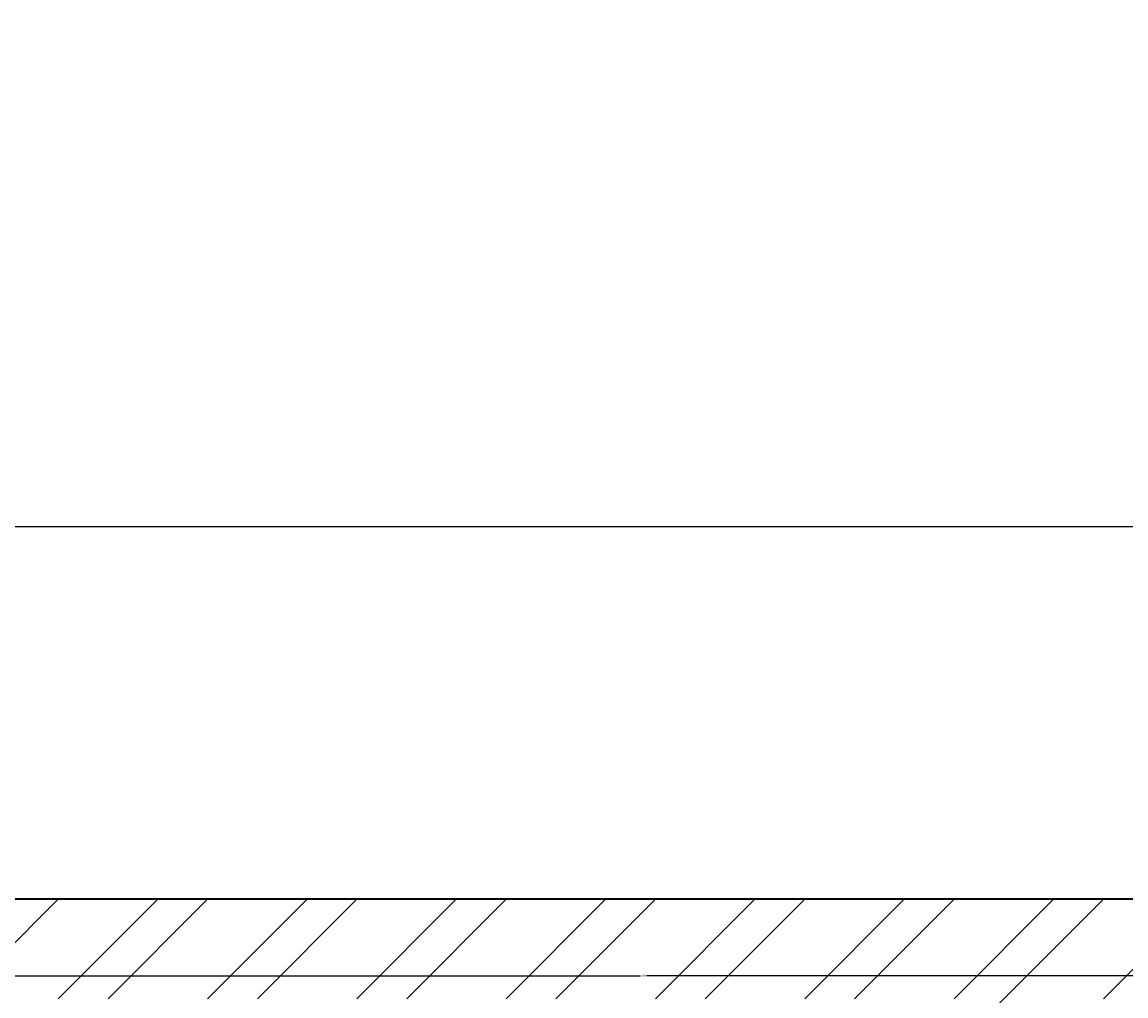
# Model space of a CAD drawing. Units: inches. Extents: x 1152 to 2588, y 1459 to 2618.
# Tile 8 of 17: x 1285 to 1384, y 2231 to 2319. Entities that reach past the tile are written whole.
import ezdxf

# ---------------------------------------------------------------- set-up
doc = ezdxf.new("R2010")
doc.units = ezdxf.units.IN
for name, color, linetype, lineweight in [('A-ANNO-DIMS', 2, 'Continuous', 18), ('A-WALL', 7, 'Continuous', 35), ('A-WALL-PATT', 8, 'Continuous', 13)]:
    doc.layers.add(name, color=color, linetype=linetype, lineweight=lineweight)
doc.styles.get("Standard").update_dxf_attribs({"font": 'arial.ttf'})
doc.dimstyles.get("Standard").update_dxf_attribs({"dimtxt": 0.18, "dimasz": 0.18, "dimexe": 0.18, "dimexo": 0.0625, "dimgap": 0.09, "dimtad": 0, "dimtih": 1, "dimtoh": 1, "dimdec": 4, "dimzin": 0, "dimdsep": 46, "dimtxsty": 'Standard', "dimcen": 0.09, "dimadec": 0, "dimazin": 0, "dimtfac": 1, "dimtdec": 4, "dimtofl": 0, "dimtmove": 0, "dimatfit": 3, "dimfxl": 1, "dimtolj": 1, "dimtzin": 0, "dimarcsym": 0})

# ---------------------------------------------------------------- blocks, each defined once
blk = doc.blocks.new('*D70')
at = {"layer": 'A-ANNO-DIMS', "color": 0, "lineweight": -2, "transparency": 16777216}
for p, q in [((1276.417, 2240.108), (1276.417, 2273.826)), ((1276.597, 2273.646), (1506.124, 2273.646)), ((1736.237, 2273.646), (1506.709, 2273.646)), ((1736.417, 2240.108), (1736.417, 2273.826))]:
    blk.add_line(p, q, dxfattribs=at)
at = {"layer": 'A-ANNO-DIMS', "color": 0, "transparency": 16777216}
for points in [[(1276.597, 2273.676), (1276.597, 2273.616), (1276.417, 2273.646)], [(1736.237, 2273.676), (1736.237, 2273.616), (1736.417, 2273.646)]]:
    blk.add_solid(points, dxfattribs=at)
at = {"layer": 'Defpoints', "color": 0, "transparency": 16777216}
for p in [(1736.417, 2273.646), (1276.417, 2240.046), (1736.417, 2240.046)]:
    blk.add_point(p, dxfattribs=at)
at = {"layer": 'A-ANNO-DIMS', "color": 0, "transparency": 16777216, "insert": (1506.417, 2273.646), "char_height": 0.18, "attachment_point": 5}
blk.add_mtext('\\A1;460', dxfattribs=at)
blk = doc.blocks.new('*D91')
at = {"layer": 'A-ANNO-DIMS', "color": 0, "lineweight": -2, "transparency": 16777216}
for p, q in [((1405.417, 2327.329), (1405.417, 2232.94)), ((1276.417, 2321.329), (1276.417, 2232.94)), ((1276.597, 2233.12), (1340.636, 2233.12)), ((1405.237, 2233.12), (1341.197, 2233.12))]:
    blk.add_line(p, q, dxfattribs=at)
at = {"layer": 'A-ANNO-DIMS', "color": 0, "transparency": 16777216}
for points in [[(1276.597, 2233.15), (1276.597, 2233.09), (1276.417, 2233.12)], [(1405.237, 2233.15), (1405.237, 2233.09), (1405.417, 2233.12)]]:
    blk.add_solid(points, dxfattribs=at)
at = {"layer": 'Defpoints', "color": 0, "transparency": 16777216}
for p in [(1405.417, 2327.391), (1276.417, 2321.391), (1405.417, 2233.12)]:
    blk.add_point(p, dxfattribs=at)
at = {"layer": 'A-ANNO-DIMS', "color": 0, "transparency": 16777216, "insert": (1340.917, 2233.12), "char_height": 0.18, "attachment_point": 5}
blk.add_mtext('\\A1;129', dxfattribs=at)

msp = doc.modelspace()

# ---------------------------------------------------------------- hatches: boundary and pattern name
at = {"layer": 'A-WALL-PATT'}
h = msp.add_hatch(dxfattribs=at)
h.set_pattern_fill('ANSI32', color=256)
h.paths.add_polyline_path([(1408.9272, 2240.0458), (1276.4165, 2240.0458), (1276.4165, 2192.7491), (1285.4165, 2192.7491), (1285.4165, 2231.0458), (1369.4165, 2231.0458), (1369.4165, 2084.0458), (1526.9165, 2084.0458), (1526.9165, 2096.3728), (1524.6665, 2096.3728), (1522.4165, 2096.3728), (1522.4165, 2093.0458), (1378.4165, 2093.0458), (1378.4165, 2231.0458), (1408.9272, 2231.0458)])
h.paths.add_polyline_path([(1736.4165, 2240.0458), (1468.9272, 2240.0458), (1468.9272, 2231.0458), (1522.4165, 2231.0458), (1522.4165, 2127.3313), (1526.9165, 2127.3313), (1526.9165, 2231.0458), (1574.9165, 2231.0458), (1574.9165, 2188.0458), (1579.4165, 2188.0458), (1579.4165, 2231.0458), (1727.4165, 2231.0458), (1727.4165, 2183.9728), (1736.4165, 2183.9728)])
h.paths.add_polyline_path([(1285.4165, 2156.7491), (1276.4165, 2156.7491), (1276.4165, 2084.0458), (1285.4165, 2084.0458)], flags=17)
h.paths.add_polyline_path([(1285.4165, 2043.5458), (1445.4165, 2043.5458), (1445.4165, 1943.6503), (1454.4165, 1943.6503), (1454.4165, 2048.0458), (1276.4165, 2048.0458), (1276.4165, 2019.2077), (1280.9165, 2019.2077), (1285.4165, 2019.2077)])
h.paths.add_polyline_path([(1285.4165, 1959.2077), (1276.4165, 1959.2077), (1276.4165, 1891.1319), (1280.9165, 1891.1319), (1285.4165, 1891.1319), (1285.4165, 1901.0458), (1376.8505, 1901.0458), (1376.8505, 1903.2958), (1376.8505, 1905.5458), (1285.4165, 1905.5458)])
h.paths.add_polyline_path([(1518.4165, 1905.5458), (1399.2832, 1905.5458), (1399.2832, 1903.2958), (1399.2832, 1901.0458), (1405.4165, 1901.0458), (1405.4165, 1884.8579), (1409.9165, 1884.8579), (1409.9165, 1901.0458), (1513.9165, 1901.0458), (1513.9165, 1869.1706), (1518.4165, 1869.1706)])
h.paths.add_polyline_path([(1520.5229, 1845.0458), (1518.4165, 1845.0458), (1518.4165, 1849.2927), (1516.1665, 1849.2927), (1513.9165, 1849.2927), (1513.9165, 1845.0458), (1409.9165, 1845.0458), (1409.9165, 1860.8579), (1405.4165, 1860.8579), (1405.4165, 1845.0458), (1285.4165, 1845.0458), (1285.4165, 1867.1319), (1276.4165, 1867.1319), (1276.4165, 1635.0458), (1285.4165, 1635.0458), (1285.4165, 1836.0458), (1405.4165, 1836.0458), (1405.4165, 1635.0458), (1414.4165, 1635.0458), (1424.7277, 1635.0458), (1424.7277, 1639.5458), (1424.7277, 1644.0458), (1414.4165, 1644.0458), (1414.4165, 1836.0458), (1414.4165, 1840.5831), (1520.5229, 1840.5831)])
h.paths.add_polyline_path([(1579.4165, 1840.5458), (1583.4035, 1840.5458), (1583.4035, 1845.0458), (1579.4165, 1845.0458), (1570.4165, 1845.0458), (1570.4165, 1840.5831), (1570.4165, 1644.0458), (1548.2359, 1644.0458), (1548.2359, 1635.0458), (1611.2801, 1635.0458), (1611.2801, 1639.5458), (1611.2801, 1644.0458), (1579.4165, 1644.0458)])
h.paths.add_polyline_path([(1488.2359, 1644.0458), (1472.0663, 1644.0458), (1472.0663, 1635.0458), (1488.2359, 1635.0458), (1488.2359, 1639.5458)], flags=17)
h.paths.add_polyline_path([(1736.4165, 1701.1863), (1727.4165, 1701.1863), (1727.4165, 1644.0458), (1671.2801, 1644.0458), (1671.2801, 1635.0458), (1736.4165, 1635.0458)])
h.paths.add_polyline_path([(1736.4165, 2147.9728), (1727.4165, 2147.9728), (1727.4165, 2093.0458), (1579.4165, 2093.0458), (1574.9165, 2093.0458), (1574.9165, 1971.6501), (1579.4165, 1971.6501), (1579.4165, 2084.0458), (1727.4165, 2084.0458), (1727.4165, 2054.3847), (1736.4165, 2054.3847)])
h.paths.add_polyline_path([(1736.4165, 1994.3847), (1727.4165, 1994.3847), (1727.4165, 1911.3562), (1736.4165, 1911.3562)])
h.paths.add_polyline_path([(1736.4165, 1875.3562), (1727.4165, 1875.3562), (1727.4165, 1845.0458), (1617.1767, 1845.0458), (1617.1767, 1842.7958), (1617.1767, 1840.5458), (1618.9165, 1840.5458), (1618.9165, 1788.5458), (1618.9165, 1784.0458), (1627.8699, 1784.0458), (1627.8699, 1788.5458), (1623.4165, 1788.5458), (1623.4165, 1840.5458), (1727.4165, 1840.5458), (1727.4165, 1828.7619), (1736.4165, 1828.7619)])
h.paths.add_polyline_path([(1727.4165, 1938.0458), (1579.4165, 1938.0458), (1579.4165, 1942.7722), (1574.9165, 1942.7722), (1574.9165, 1929.0458), (1727.4165, 1929.0458)])

# ---------------------------------------------------------------- linework, layer by layer
at = {"layer": 'A-WALL'}
msp.add_line((1276.4165, 2240.0458), (1736.4165, 2240.0458), dxfattribs=at)

# ---------------------------------------------------------------- dimensions: what is measured, and where the dimension line sits
at = {"layer": 'A-ANNO-DIMS'}
for base, p1, p2, picture, middle in [((1405.4165, 2233.12), (1276.4165, 2321.3911), (1405.4165, 2327.3911), '*D91', (1340.9165, 2233.12)), ((1736.4165, 2273.6458), (1276.4165, 2240.0458), (1736.4165, 2240.0458), '*D70', (1506.4165, 2273.6458))]:
    dim = msp.add_linear_dim(base=base, p1=p1, p2=p2, dimstyle='Standard', override={"dimdec": 0, "dimlfac": 1, "dimrnd": 0, "dimzin": 0, "dimdsep": 46, "dimlunit": 2}, dxfattribs=at)
    dim.commit()
    dim.dimension.update_dxf_attribs({"geometry": picture, "text_midpoint": middle})

doc.saveas('drawing.dxf')
